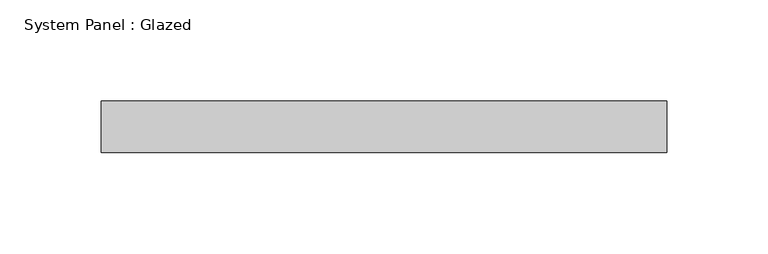
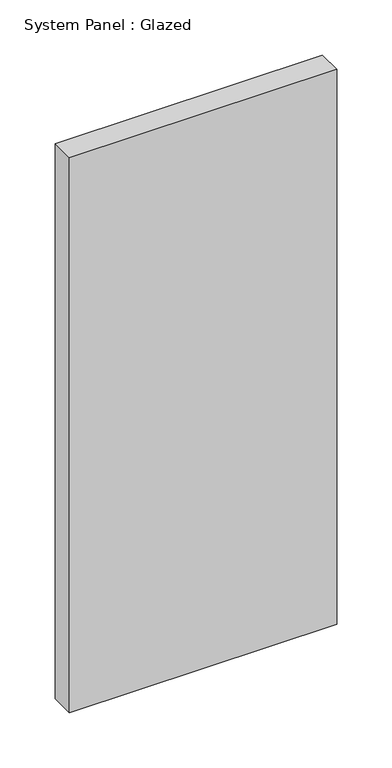
"""IFC4 building model written with IfcOpenShell, lengths in millimetres: plate geometry, System Panel : Glazed."""

from ifc_helpers import new_model, si_unit, origin, origin_with_axes, place, context, project, spatial, polyline, outline, extrude, source, transform, mapped, element, save


def system_panel_glazed_f1f3e2b8(model_context):
    return source(origin(), model_context, "Body", "SweptSolid", [
        extrude(outline(polyline([(139.7, 19.05), (-139.7, 19.05), (-139.7, 44.45), (139.7, 44.45), (139.7, 19.05)])), origin_with_axes(), (0.0, 0.0, 1.0), 613.519824),
    ])


if __name__ == "__main__":
    model = new_model("IFC4")
    model_context = context("Model", 3, world=origin())
    ifc_project = project(units=[si_unit("LENGTHUNIT", "METRE", prefix="MILLI")], contexts=[model_context])
    site = spatial("IfcSite", under=ifc_project)
    building = spatial("IfcBuilding", under=site)
    placement = place(None, origin())
    system_panel_glazed_shape = system_panel_glazed_f1f3e2b8(model_context)
    element("IfcPlate", 1, ObjectType="System Panel : Glazed", at=placement, inside=building, context=model_context, shape_type="MappedRepresentation", body=[
        mapped(system_panel_glazed_shape, transform((0.0, 0.0, 0.0), x_axis=(1.0, 0.0, 0.0), y_axis=(0.0, 1.0, 0.0), z_axis=(0.0, 0.0, 1.0))),
    ])
    save(model, "model.ifc")

# Revit data of these elements
# Type "System Panel : Glazed"
#   Construction Type Id = "GSP4R"
#   Analytic Construction = "1/8 in Pilkington single glazing"
#   Visual Light Transmittance = 0.9
#   Solar Heat Gain Coefficient = 0.86
#   Heat Transfer Coefficient (U) = 1.18115 BTU/(h·ft²·°F)
#   Define Thermal Properties by = 1
# Element 1 (IfcPlate, "System Panel : Glazed")
#   Materials on its faces: "Glass"
# Materials
#   "Glass": class "Glass", colour RGB 0 128 192, transparency 0.75, Description = "Soda Lime Glass", Cost = 0
